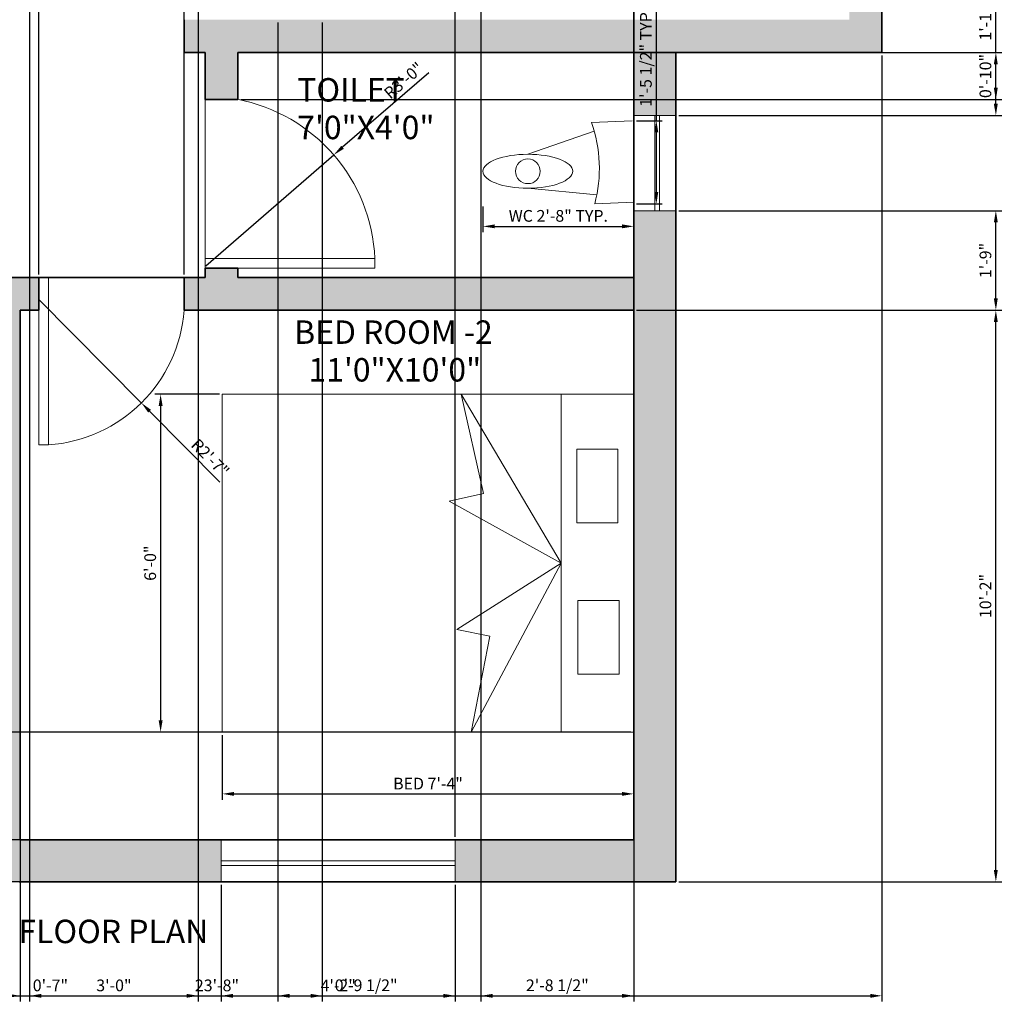
# Model space of a CAD drawing. Units: millimetres. Extents: x 2466 to 2817, y 2000 to 2512.
# Tile 2 of 4: x 2607 to 2817, y 2000 to 2210. Entities that reach past the tile are written whole.
import ezdxf

# ---------------------------------------------------------------- set-up
doc = ezdxf.new("R2010")
doc.units = ezdxf.units.MM
for name, color, linetype, lineweight in [('A-ANNO-DIMS', 2, 'Continuous', 13), ('A-ANNO-TEXT', 7, 'Continuous', 18), ('A-AREA-IDEN', 7, 'Continuous', 18), ('A-DOOR', 3, 'Continuous', 18), ('A-FLOR-FIXT', 9, 'Continuous', 18), ('A-FURN', 8, 'Continuous', 18), ('A-GLAZ', 5, 'Continuous', 18), ('A-WALL', 7, 'Continuous', 35), ('A-WALL-PATT', 8, 'Continuous', 13)]:
    doc.layers.add(name, color=color, linetype=linetype, lineweight=lineweight)
doc.styles.get("Standard").update_dxf_attribs({"font": 'arial.ttf'})
doc.dimstyles.new('ISO-25', dxfattribs={"dimtxt": 2.5, "dimasz": 2.5, "dimexe": 1.25, "dimexo": 0.625, "dimtad": 1, "dimdec": 0, "dimlunit": 3, "dimtxsty": 'Standard', "dimcen": 2.5, "dimadec": 0, "dimazin": 0, "dimtfac": 1, "dimtdec": 0, "dimtmove": 0, "dimatfit": 3, "dimfxl": 1, "dimarcsym": 0})

# ---------------------------------------------------------------- blocks, each defined once
blk = doc.blocks.new('MODERN BED')
at = {"color": 0}
for p, q in [((-79.02, 96.24), (0, 96.24)), ((-79.02, 0), (-79.02, 96.24)), ((0, 96.24), (0, 0)), ((0, 79.26), (-79.02, 79.26)), ((-39.51, 79.26), (-79.02, 55.87)), ((-53.99, 53.1), (-39.51, 79.26)), ((-39.51, 79.26), (0, 58.21)), ((-23.98, 54.83), (-39.51, 79.26)), ((-22.46, 62.6), (-23.98, 54.83)), ((0, 58.21), (-22.46, 62.6)), ((-79.02, 55.87), (-55.81, 61.13)), ((-55.81, 61.13), (-53.99, 53.1)), ((0, 0), (-79.02, 0))]:
    blk.add_line(p, q, dxfattribs=at)
for points in [[(-66.19, 92.55), (-48.93, 92.55), (-48.93, 82.91), (-66.19, 82.91)], [(-30.8, 92.85), (-13.54, 92.85), (-13.54, 83.2), (-30.8, 83.2)], [(-30.8, 92.85), (-13.54, 92.85), (-13.54, 83.2), (-30.8, 83.2)]]:
    blk.add_lwpolyline(points, close=True, dxfattribs=at)
blk = doc.blocks.new('*D10')
at = {"layer": 'A-ANNO-DIMS', "color": 0, "lineweight": -2, "transparency": 16777216}
for p, q in [((2746.56, 2482.15), (2467.98, 2482.15)), ((2469.23, 2479.65), (2469.23, 2028.65)), ((2746.56, 2026.15), (2467.98, 2026.15))]:
    blk.add_line(p, q, dxfattribs=at)
at = {"layer": 'A-ANNO-DIMS', "color": 0, "transparency": 16777216}
for points in [[(2468.82, 2479.65), (2469.65, 2479.65), (2469.23, 2482.15)], [(2468.82, 2028.65), (2469.65, 2028.65), (2469.23, 2026.15)]]:
    blk.add_solid(points, dxfattribs=at)
at = {"layer": 'Defpoints', "color": 0, "transparency": 16777216}
for p in [(2747.19, 2482.15), (2469.23, 2026.15), (2747.19, 2026.15)]:
    blk.add_point(p, dxfattribs=at)
at = {"layer": 'A-ANNO-DIMS', "color": 0, "transparency": 16777216, "insert": (2467.33, 2254.15), "char_height": 2.5, "attachment_point": 5, "rotation": 90}
blk.add_mtext("38'", dxfattribs=at)
blk = doc.blocks.new('WC-PLAN')
for p, q in [((23.15, 17.36), (31.83, 17.72)), ((23.74, 15.5), (9.57, 10.55)), ((24.29, 1.87), (9.58, 3.3)), ((32.19, 0.34), (23.86, 0))]:
    blk.add_line(p, q)
blk.add_circle((9.58, 6.93), 2.64)
blk.add_arc((-4.38, 7.53), 29.23, 345.0736, 19.6488)
blk.add_ellipse((9.58, 6.93), major_axis=(9.58, 0.01), ratio=0.378572)
blk = doc.blocks.new('WIN-BATH')
for p, q in [((4.5, 20.33), (4.5, 0)), ((5.5, 20.33), (5.5, 0))]:
    blk.add_line(p, q)
blk.add_lwpolyline([(9, 20.33), (0, 20.33), (0, 0), (9, 0)], close=True)
blk = doc.blocks.new('*D20')
at = {"layer": 'A-ANNO-DIMS', "color": 0, "lineweight": -2, "transparency": 16777216}
for p, q in [((2706, 2170.25), (2706, 2164.79)), ((2738.19, 2170.25), (2738.19, 2164.79)), ((2708.5, 2166.04), (2735.69, 2166.04))]:
    blk.add_line(p, q, dxfattribs=at)
at = {"layer": 'A-ANNO-DIMS', "color": 0, "transparency": 16777216}
for points in [[(2708.5, 2166.46), (2708.5, 2165.63), (2706, 2166.04)], [(2735.69, 2166.46), (2735.69, 2165.63), (2738.19, 2166.04)]]:
    blk.add_solid(points, dxfattribs=at)
at = {"layer": 'Defpoints', "color": 0, "transparency": 16777216}
for p in [(2706, 2170.87), (2738.19, 2170.87), (2738.19, 2166.04)]:
    blk.add_point(p, dxfattribs=at)
at = {"layer": 'A-ANNO-DIMS', "color": 0, "transparency": 16777216, "insert": (2722.09, 2167.96), "char_height": 2.5, "attachment_point": 5}
blk.add_mtext('WC 2\'-8" TYP.', dxfattribs=at)
blk = doc.blocks.new('*D21')
at = {"layer": 'A-ANNO-DIMS', "color": 0, "lineweight": -2, "transparency": 16777216}
for p, q in [((2743.02, 2188.59), (2743.02, 2213.17)), ((2738.81, 2188.59), (2744.27, 2188.59)), ((2743.02, 2173.37), (2743.02, 2186.09)), ((2738.81, 2170.87), (2744.27, 2170.87))]:
    blk.add_line(p, q, dxfattribs=at)
at = {"layer": 'A-ANNO-DIMS', "color": 0, "transparency": 16777216}
for points in [[(2742.6, 2186.09), (2743.43, 2186.09), (2743.02, 2188.59)], [(2742.6, 2173.37), (2743.43, 2173.37), (2743.02, 2170.87)]]:
    blk.add_solid(points, dxfattribs=at)
at = {"layer": 'Defpoints', "color": 0, "transparency": 16777216}
for p in [(2738.19, 2188.59), (2743.02, 2188.59), (2738.19, 2170.87)]:
    blk.add_point(p, dxfattribs=at)
at = {"layer": 'A-ANNO-DIMS', "color": 0, "transparency": 16777216, "insert": (2741.1, 2202.13), "char_height": 2.5, "attachment_point": 5, "rotation": 90}
blk.add_mtext('1\'-5 1/2" TYP.', dxfattribs=at)
blk = doc.blocks.new('*D22')
at = {"layer": 'A-ANNO-DIMS', "color": 0, "lineweight": -2, "transparency": 16777216}
for p, q in [((2650.34, 2057.48), (2650.34, 2043.67)), ((2738.19, 2057.48), (2738.19, 2043.67)), ((2652.84, 2044.92), (2735.69, 2044.92))]:
    blk.add_line(p, q, dxfattribs=at)
at = {"layer": 'A-ANNO-DIMS', "color": 0, "transparency": 16777216}
for points in [[(2652.84, 2045.34), (2652.84, 2044.51), (2650.34, 2044.92)], [(2735.69, 2045.34), (2735.69, 2044.51), (2738.19, 2044.92)]]:
    blk.add_solid(points, dxfattribs=at)
at = {"layer": 'Defpoints', "color": 0, "transparency": 16777216}
for p in [(2650.34, 2058.1), (2738.19, 2058.1), (2738.19, 2044.92)]:
    blk.add_point(p, dxfattribs=at)
at = {"layer": 'A-ANNO-DIMS', "color": 0, "transparency": 16777216, "insert": (2694.26, 2046.8), "char_height": 2.5, "attachment_point": 5}
blk.add_mtext('BED 7\'-4"', dxfattribs=at)
blk = doc.blocks.new('*D23')
at = {"layer": 'A-ANNO-DIMS', "color": 0, "lineweight": -2, "transparency": 16777216}
for p, q in [((2649.72, 2130.23), (2635.91, 2130.23)), ((2637.16, 2127.73), (2637.16, 2060.6)), ((2649.72, 2058.1), (2635.91, 2058.1))]:
    blk.add_line(p, q, dxfattribs=at)
at = {"layer": 'A-ANNO-DIMS', "color": 0, "transparency": 16777216}
for points in [[(2636.75, 2127.73), (2637.58, 2127.73), (2637.16, 2130.23)], [(2636.75, 2060.6), (2637.58, 2060.6), (2637.16, 2058.1)]]:
    blk.add_solid(points, dxfattribs=at)
at = {"layer": 'Defpoints', "color": 0, "transparency": 16777216}
for p in [(2650.34, 2130.23), (2637.16, 2058.1), (2650.34, 2058.1)]:
    blk.add_point(p, dxfattribs=at)
at = {"layer": 'A-ANNO-DIMS', "color": 0, "transparency": 16777216, "insert": (2635.26, 2094.16), "char_height": 2.5, "attachment_point": 5, "rotation": 90}
blk.add_mtext('6\'-0"', dxfattribs=at)
blk = doc.blocks.new('*D26')
at = {"layer": 'A-ANNO-DIMS', "color": 0, "lineweight": -2, "transparency": 16777216}
for p, q in [((2791.19, 2202.52), (2791.19, 2000.58)), ((2507.19, 2047.52), (2507.19, 2000.58)), ((2509.69, 2001.83), (2788.69, 2001.83))]:
    blk.add_line(p, q, dxfattribs=at)
at = {"layer": 'A-ANNO-DIMS', "color": 0, "transparency": 16777216}
for points in [[(2509.69, 2002.24), (2509.69, 2001.41), (2507.19, 2001.83)], [(2788.69, 2002.24), (2788.69, 2001.41), (2791.19, 2001.83)]]:
    blk.add_solid(points, dxfattribs=at)
at = {"layer": 'Defpoints', "color": 0, "transparency": 16777216}
for p in [(2791.19, 2203.15), (2507.19, 2048.15), (2791.19, 2001.83)]:
    blk.add_point(p, dxfattribs=at)
at = {"layer": 'A-ANNO-DIMS', "color": 0, "transparency": 16777216, "insert": (2649.19, 2003.73), "char_height": 2.5, "attachment_point": 5}
blk.add_mtext('23\'-8"', dxfattribs=at)
blk = doc.blocks.new('*D42')
at = {"layer": 'A-ANNO-DIMS', "color": 0, "lineweight": -2, "transparency": 16777216}
for p, q in [((2650.11, 2025.52), (2650.11, 2000.58)), ((2700.05, 2025.52), (2700.05, 2000.58)), ((2652.61, 2001.83), (2697.55, 2001.83))]:
    blk.add_line(p, q, dxfattribs=at)
at = {"layer": 'A-ANNO-DIMS', "color": 0, "transparency": 16777216}
for points in [[(2652.61, 2002.24), (2652.61, 2001.41), (2650.11, 2001.83)], [(2697.55, 2002.24), (2697.55, 2001.41), (2700.05, 2001.83)]]:
    blk.add_solid(points, dxfattribs=at)
at = {"layer": 'Defpoints', "color": 0, "transparency": 16777216}
for p in [(2650.11, 2026.15), (2700.05, 2026.15), (2700.05, 2001.83)]:
    blk.add_point(p, dxfattribs=at)
at = {"layer": 'A-ANNO-DIMS', "color": 0, "transparency": 16777216, "insert": (2675.08, 2003.71), "char_height": 2.5, "attachment_point": 5}
blk.add_mtext('4\'-2"', dxfattribs=at)
blk = doc.blocks.new('*D43')
at = {"layer": 'A-ANNO-DIMS', "color": 0, "lineweight": -2, "transparency": 16777216}
for p, q in [((2700.05, 2035.77), (2700.05, 2507.72)), ((2702.55, 2506.47), (2735.69, 2506.47)), ((2738.19, 2035.77), (2738.19, 2507.72))]:
    blk.add_line(p, q, dxfattribs=at)
at = {"layer": 'A-ANNO-DIMS', "color": 0, "transparency": 16777216}
for points in [[(2702.55, 2506.88), (2702.55, 2506.05), (2700.05, 2506.47)], [(2735.69, 2506.88), (2735.69, 2506.05), (2738.19, 2506.47)]]:
    blk.add_solid(points, dxfattribs=at)
at = {"layer": 'Defpoints', "color": 0, "transparency": 16777216}
for p in [(2738.19, 2506.47), (2700.05, 2035.15), (2738.19, 2035.15)]:
    blk.add_point(p, dxfattribs=at)
at = {"layer": 'A-ANNO-DIMS', "color": 0, "transparency": 16777216, "insert": (2719.12, 2508.37), "char_height": 2.5, "attachment_point": 5}
blk.add_mtext('3\'-2"', dxfattribs=at)
blk = doc.blocks.new('*D50')
at = {"layer": 'A-ANNO-DIMS', "color": 0, "lineweight": -2, "transparency": 16777216}
for p, q in [((2609.19, 2348.52), (2609.19, 2000.58)), ((2645.19, 2348.52), (2645.19, 2000.58)), ((2611.69, 2001.83), (2642.69, 2001.83))]:
    blk.add_line(p, q, dxfattribs=at)
at = {"layer": 'A-ANNO-DIMS', "color": 0, "transparency": 16777216}
for points in [[(2611.69, 2002.24), (2611.69, 2001.41), (2609.19, 2001.83)], [(2642.69, 2002.24), (2642.69, 2001.41), (2645.19, 2001.83)]]:
    blk.add_solid(points, dxfattribs=at)
at = {"layer": 'Defpoints', "color": 0, "transparency": 16777216}
for p in [(2609.19, 2349.15), (2645.19, 2349.15), (2645.19, 2001.83)]:
    blk.add_point(p, dxfattribs=at)
at = {"layer": 'A-ANNO-DIMS', "color": 0, "transparency": 16777216, "insert": (2627.19, 2003.73), "char_height": 2.5, "attachment_point": 5}
blk.add_mtext('3\'-0"', dxfattribs=at)
blk = doc.blocks.new('*D53')
at = {"layer": 'A-ANNO-DIMS', "color": 0, "lineweight": -2, "transparency": 16777216}
for p, q in [((2596.19, 2155.77), (2596.19, 2507.72)), ((2598.69, 2506.47), (2608.69, 2506.47)), ((2611.19, 2155.77), (2611.19, 2507.72))]:
    blk.add_line(p, q, dxfattribs=at)
at = {"layer": 'A-ANNO-DIMS', "color": 0, "transparency": 16777216}
for points in [[(2598.69, 2506.88), (2598.69, 2506.05), (2596.19, 2506.47)], [(2608.69, 2506.88), (2608.69, 2506.05), (2611.19, 2506.47)]]:
    blk.add_solid(points, dxfattribs=at)
at = {"layer": 'Defpoints', "color": 0, "transparency": 16777216}
for p in [(2611.19, 2506.47), (2596.19, 2155.15), (2611.19, 2155.15)]:
    blk.add_point(p, dxfattribs=at)
at = {"layer": 'A-ANNO-DIMS', "color": 0, "transparency": 16777216, "insert": (2603.69, 2508.37), "char_height": 2.5, "attachment_point": 5}
blk.add_mtext('1\'-3"', dxfattribs=at)
blk = doc.blocks.new('*D54')
at = {"layer": 'A-ANNO-DIMS', "color": 0, "lineweight": -2, "transparency": 16777216}
for p, q in [((2611.19, 2155.77), (2611.19, 2507.72)), ((2613.69, 2506.47), (2639.69, 2506.47)), ((2642.19, 2155.77), (2642.19, 2507.72))]:
    blk.add_line(p, q, dxfattribs=at)
at = {"layer": 'A-ANNO-DIMS', "color": 0, "transparency": 16777216}
for points in [[(2613.69, 2506.88), (2613.69, 2506.05), (2611.19, 2506.47)], [(2639.69, 2506.88), (2639.69, 2506.05), (2642.19, 2506.47)]]:
    blk.add_solid(points, dxfattribs=at)
at = {"layer": 'Defpoints', "color": 0, "transparency": 16777216}
for p in [(2642.19, 2506.47), (2611.19, 2155.15), (2642.19, 2155.15)]:
    blk.add_point(p, dxfattribs=at)
at = {"layer": 'A-ANNO-DIMS', "color": 0, "transparency": 16777216, "insert": (2626.69, 2508.35), "char_height": 2.5, "attachment_point": 5}
blk.add_mtext('2\'-7"', dxfattribs=at)
blk = doc.blocks.new('*D55')
at = {"layer": 'A-ANNO-DIMS', "color": 0, "lineweight": -2, "transparency": 16777216}
for p, q in [((2738.81, 2148.15), (2816.76, 2148.15)), ((2815.51, 2028.65), (2815.51, 2145.65)), ((2747.81, 2026.15), (2816.76, 2026.15))]:
    blk.add_line(p, q, dxfattribs=at)
at = {"layer": 'A-ANNO-DIMS', "color": 0, "transparency": 16777216}
for points in [[(2815.09, 2145.65), (2815.92, 2145.65), (2815.51, 2148.15)], [(2815.09, 2028.65), (2815.92, 2028.65), (2815.51, 2026.15)]]:
    blk.add_solid(points, dxfattribs=at)
at = {"layer": 'Defpoints', "color": 0, "transparency": 16777216}
for p in [(2738.19, 2148.15), (2815.51, 2148.15), (2747.19, 2026.15)]:
    blk.add_point(p, dxfattribs=at)
at = {"layer": 'A-ANNO-DIMS', "color": 0, "transparency": 16777216, "insert": (2813.61, 2087.15), "char_height": 2.5, "attachment_point": 5, "rotation": 90}
blk.add_mtext('10\'-2"', dxfattribs=at)
blk = doc.blocks.new('*D56')
at = {"layer": 'A-ANNO-DIMS', "color": 0, "lineweight": -2, "transparency": 16777216}
for p, q in [((2747.81, 2169.38), (2816.76, 2169.38)), ((2815.51, 2150.65), (2815.51, 2166.88)), ((2738.81, 2148.15), (2816.76, 2148.15))]:
    blk.add_line(p, q, dxfattribs=at)
at = {"layer": 'A-ANNO-DIMS', "color": 0, "transparency": 16777216}
for points in [[(2815.09, 2166.88), (2815.92, 2166.88), (2815.51, 2169.38)], [(2815.09, 2150.65), (2815.92, 2150.65), (2815.51, 2148.15)]]:
    blk.add_solid(points, dxfattribs=at)
at = {"layer": 'Defpoints', "color": 0, "transparency": 16777216}
for p in [(2747.19, 2169.38), (2815.51, 2169.38), (2738.19, 2148.15)]:
    blk.add_point(p, dxfattribs=at)
at = {"layer": 'A-ANNO-DIMS', "color": 0, "transparency": 16777216, "insert": (2813.61, 2158.76), "char_height": 2.5, "attachment_point": 5, "rotation": 90}
blk.add_mtext('1\'-9"', dxfattribs=at)
blk = doc.blocks.new('*D57')
at = {"layer": 'A-ANNO-DIMS', "color": 0, "lineweight": -2, "transparency": 16777216}
for p, q in [((2815.51, 2203.15), (2815.51, 2219.13)), ((2747.81, 2203.15), (2816.76, 2203.15)), ((2815.51, 2192.2), (2815.51, 2200.65)), ((2747.81, 2189.7), (2816.76, 2189.7))]:
    blk.add_line(p, q, dxfattribs=at)
at = {"layer": 'A-ANNO-DIMS', "color": 0, "transparency": 16777216}
for points in [[(2815.09, 2200.65), (2815.92, 2200.65), (2815.51, 2203.15)], [(2815.09, 2192.2), (2815.92, 2192.2), (2815.51, 2189.7)]]:
    blk.add_solid(points, dxfattribs=at)
at = {"layer": 'Defpoints', "color": 0, "transparency": 16777216}
for p in [(2747.19, 2203.15), (2815.51, 2203.15), (2747.19, 2189.7)]:
    blk.add_point(p, dxfattribs=at)
at = {"layer": 'A-ANNO-DIMS', "color": 0, "transparency": 16777216, "insert": (2813.59, 2212.39), "char_height": 2.5, "attachment_point": 5, "rotation": 90}
blk.add_mtext('1\'-1 1/2"', dxfattribs=at)
blk = doc.blocks.new('*D59')
at = {"layer": 'A-ANNO-DIMS', "color": 0, "lineweight": -2, "transparency": 16777216}
for p, q in [((2600.19, 2147.52), (2600.19, 2000.58)), ((2607.19, 2147.52), (2607.19, 2000.58)), ((2602.69, 2001.83), (2604.69, 2001.83)), ((2607.19, 2001.83), (2617.58, 2001.83))]:
    blk.add_line(p, q, dxfattribs=at)
at = {"layer": 'A-ANNO-DIMS', "color": 0, "transparency": 16777216}
for points in [[(2602.69, 2002.24), (2602.69, 2001.41), (2600.19, 2001.83)], [(2604.69, 2002.24), (2604.69, 2001.41), (2607.19, 2001.83)]]:
    blk.add_solid(points, dxfattribs=at)
at = {"layer": 'Defpoints', "color": 0, "transparency": 16777216}
for p in [(2600.19, 2148.15), (2607.19, 2148.15), (2607.19, 2001.83)]:
    blk.add_point(p, dxfattribs=at)
at = {"layer": 'A-ANNO-DIMS', "color": 0, "transparency": 16777216, "insert": (2613.63, 2003.73), "char_height": 2.5, "attachment_point": 5}
blk.add_mtext('0\'-7"', dxfattribs=at)
blk = doc.blocks.new('*D62')
at = {"layer": 'A-ANNO-DIMS', "color": 0, "lineweight": -2, "transparency": 16777216}
for p, q in [((2654.3, 2203.15), (2816.76, 2203.15)), ((2815.51, 2195.61), (2815.51, 2200.65)), ((2654.3, 2193.11), (2816.76, 2193.11))]:
    blk.add_line(p, q, dxfattribs=at)
at = {"layer": 'A-ANNO-DIMS', "color": 0, "transparency": 16777216}
for points in [[(2815.09, 2200.65), (2815.92, 2200.65), (2815.51, 2203.15)], [(2815.09, 2195.61), (2815.92, 2195.61), (2815.51, 2193.11)]]:
    blk.add_solid(points, dxfattribs=at)
at = {"layer": 'Defpoints', "color": 0, "transparency": 16777216}
for p in [(2653.68, 2203.15), (2815.51, 2203.15), (2653.68, 2193.11)]:
    blk.add_point(p, dxfattribs=at)
at = {"layer": 'A-ANNO-DIMS', "color": 0, "transparency": 16777216, "insert": (2813.61, 2198.13), "char_height": 2.5, "attachment_point": 5, "rotation": 90}
blk.add_mtext('0\'-10"', dxfattribs=at)
blk = doc.blocks.new('*D63')
at = {"layer": 'A-ANNO-DIMS', "color": 0, "lineweight": -2, "transparency": 16777216}
for p, q in [((2662.19, 2209.52), (2662.19, 2000.58)), ((2671.69, 2209.52), (2671.69, 2000.58)), ((2664.69, 2001.83), (2669.19, 2001.83)), ((2671.69, 2001.83), (2687.91, 2001.83))]:
    blk.add_line(p, q, dxfattribs=at)
at = {"layer": 'A-ANNO-DIMS', "color": 0, "transparency": 16777216}
for points in [[(2664.69, 2002.24), (2664.69, 2001.41), (2662.19, 2001.83)], [(2669.19, 2002.24), (2669.19, 2001.41), (2671.69, 2001.83)]]:
    blk.add_solid(points, dxfattribs=at)
at = {"layer": 'Defpoints', "color": 0, "transparency": 16777216}
for p in [(2662.19, 2210.15), (2671.69, 2210.15), (2671.69, 2001.83)]:
    blk.add_point(p, dxfattribs=at)
at = {"layer": 'A-ANNO-DIMS', "color": 0, "transparency": 16777216, "insert": (2681.05, 2003.75), "char_height": 2.5, "attachment_point": 5}
blk.add_mtext('0\'-9 1/2"', dxfattribs=at)
blk = doc.blocks.new('*D67')
at = {"layer": 'A-ANNO-DIMS', "color": 0, "lineweight": -2, "transparency": 16777216}
for p, q in [((2705.56, 2472.66), (2705.56, 2000.58)), ((2738.19, 2472.52), (2738.19, 2000.58)), ((2708.06, 2001.83), (2735.69, 2001.83))]:
    blk.add_line(p, q, dxfattribs=at)
at = {"layer": 'A-ANNO-DIMS', "color": 0, "transparency": 16777216}
for points in [[(2708.06, 2002.24), (2708.06, 2001.41), (2705.56, 2001.83)], [(2735.69, 2002.24), (2735.69, 2001.41), (2738.19, 2001.83)]]:
    blk.add_solid(points, dxfattribs=at)
at = {"layer": 'Defpoints', "color": 0, "transparency": 16777216}
for p in [(2705.56, 2473.28), (2738.19, 2473.15), (2738.19, 2001.83)]:
    blk.add_point(p, dxfattribs=at)
at = {"layer": 'A-ANNO-DIMS', "color": 0, "transparency": 16777216, "insert": (2721.87, 2003.75), "char_height": 2.5, "attachment_point": 5}
blk.add_mtext('2\'-8 1/2"', dxfattribs=at)
blk = doc.blocks.new('*D68')
at = {"layer": 'A-ANNO-DIMS', "color": 0, "lineweight": -2, "transparency": 16777216}
for p, q in [((2737.56, 2058.1), (2481.62, 2058.1)), ((2482.87, 2037.65), (2482.87, 2055.6)), ((2737.56, 2035.15), (2481.62, 2035.15))]:
    blk.add_line(p, q, dxfattribs=at)
at = {"layer": 'A-ANNO-DIMS', "color": 0, "transparency": 16777216}
for points in [[(2482.45, 2055.6), (2483.28, 2055.6), (2482.87, 2058.1)], [(2482.45, 2037.65), (2483.28, 2037.65), (2482.87, 2035.15)]]:
    blk.add_solid(points, dxfattribs=at)
at = {"layer": 'Defpoints', "color": 0, "transparency": 16777216}
for p in [(2482.87, 2058.1), (2738.19, 2058.1), (2738.19, 2035.15)]:
    blk.add_point(p, dxfattribs=at)
at = {"layer": 'A-ANNO-DIMS', "color": 0, "transparency": 16777216, "insert": (2480.99, 2046.62), "char_height": 2.5, "attachment_point": 5, "rotation": 90}
blk.add_mtext('1\'-11"', dxfattribs=at)
blk = doc.blocks.new('*D75')
at = {"layer": 'A-ANNO-DIMS', "color": 0, "lineweight": -2, "transparency": 16777216}
for p, q in [((2694.41, 2198.84), (2676.01, 2182.92)), ((2646.79, 2157.63), (2674.12, 2181.28))]:
    blk.add_line(p, q, dxfattribs=at)
at = {"layer": 'A-ANNO-DIMS', "color": 0, "transparency": 16777216}
blk.add_solid([(2675.74, 2183.23), (2676.28, 2182.6), (2674.12, 2181.28)], dxfattribs=at)
at = {"layer": 'Defpoints', "color": 0, "transparency": 16777216}
for p in [(2674.12, 2181.28), (2646.79, 2157.63)]:
    blk.add_point(p, dxfattribs=at)
at = {"layer": 'A-ANNO-DIMS', "color": 0, "transparency": 16777216, "insert": (2689.28, 2196.91), "char_height": 2.5, "attachment_point": 5, "rotation": 40.8737}
blk.add_mtext('R3\'-0"', dxfattribs=at)
blk = doc.blocks.new('*D79')
at = {"layer": 'A-ANNO-DIMS', "color": 0, "lineweight": -2, "transparency": 16777216}
for p, q in [((2611.1, 2150.52), (2633.04, 2128.38)), ((2649.83, 2111.43), (2634.8, 2126.6))]:
    blk.add_line(p, q, dxfattribs=at)
at = {"layer": 'A-ANNO-DIMS', "color": 0, "transparency": 16777216}
blk.add_solid([(2635.1, 2126.89), (2634.51, 2126.31), (2633.04, 2128.38)], dxfattribs=at)
at = {"layer": 'Defpoints', "color": 0, "transparency": 16777216}
for p in [(2611.1, 2150.52), (2633.04, 2128.38)]:
    blk.add_point(p, dxfattribs=at)
at = {"layer": 'A-ANNO-DIMS', "color": 0, "transparency": 16777216, "insert": (2647.54, 2116.41), "char_height": 2.5, "attachment_point": 5, "rotation": 314.7339}
blk.add_mtext('R2\'-7"', dxfattribs=at)

msp = doc.modelspace()

# ---------------------------------------------------------------- hatches: boundary and pattern name
at = {"layer": 'A-WALL-PATT'}
h = msp.add_hatch(color=256, dxfattribs=at)
h.dxf.hatch_style = 1
h.paths.add_polyline_path([(2791.19, 2301.15), (2747.19, 2301.15), (2747.19, 2294.15), (2784.19, 2294.15), (2784.19, 2279.03), (2791.19, 2279.03)])
h.paths.add_polyline_path([(2791.19, 2216.9), (2784.19, 2216.9), (2784.19, 2210.15), (2662.19, 2210.15), (2647.19, 2210.15), (2645.19, 2210.15), (2642.19, 2210.15), (2642.19, 2203.15), (2646.68, 2203.15), (2646.68, 2193.15), (2653.68, 2193.15), (2653.68, 2203.15), (2654.69, 2203.15), (2662.19, 2203.15), (2791.19, 2203.15)])
h = msp.add_hatch(color=256, dxfattribs=at)
h.dxf.hatch_style = 1
h.paths.add_polyline_path([(2747.19, 2203.15), (2738.19, 2203.15), (2738.19, 2189.7), (2747.19, 2189.7)])
h = msp.add_hatch(color=256, dxfattribs=at)
h.dxf.hatch_style = 1
h.paths.add_polyline_path([(2747.19, 2169.38), (2738.19, 2169.38), (2738.19, 2035.15), (2700.05, 2035.15), (2700.05, 2026.15), (2747.19, 2026.15)])
h = msp.add_hatch(color=256, dxfattribs=at)
h.dxf.hatch_style = 1
h.paths.add_polyline_path([(2516.19, 2159.02), (2507.19, 2159.02), (2507.19, 2119.17), (2516.19, 2119.17)])
h.paths.add_polyline_path([(2516.19, 2068.93), (2507.19, 2068.93), (2507.19, 2048.15), (2516.19, 2048.15), (2562.24, 2048.15), (2562.24, 2055.15), (2551.24, 2055.15), (2516.19, 2055.15)])
h.paths.add_polyline_path([(2607.19, 2148.15), (2611.19, 2148.15), (2611.19, 2155.15), (2596.19, 2155.15), (2596.19, 2148.15), (2600.19, 2148.15), (2600.19, 2055.15), (2598.12, 2055.15), (2598.12, 2048.15), (2600.19, 2048.15), (2600.19, 2035.15), (2600.19, 2026.15), (2606.96, 2026.15), (2650.11, 2026.15), (2650.11, 2035.15), (2607.19, 2035.15)])
h = msp.add_hatch(color=256, dxfattribs=at)
h.dxf.hatch_style = 1
h.paths.add_polyline_path([(2738.19, 2155.15), (2653.68, 2155.15), (2653.68, 2157.15), (2646.68, 2157.15), (2646.68, 2155.15), (2642.19, 2155.15), (2642.19, 2148.15), (2738.19, 2148.15)])

# ---------------------------------------------------------------- linework, layer by layer
at = {"layer": 'A-DOOR'}
for p, q in [((2646.7, 2157.15), (2646.68, 2193.15)), ((2682.9, 2159.15), (2646.7, 2159.15)), ((2646.7, 2159.15), (2646.7, 2157.15)), ((2653.68, 2157.15), (2682.9, 2157.15)), ((2682.9, 2157.15), (2682.9, 2159.15)), ((2613.19, 2119.42), (2613.19, 2155.15)), ((2611.19, 2148.15), (2611.19, 2119.42)), ((2611.19, 2119.42), (2613.19, 2119.42))]:
    msp.add_line(p, q, dxfattribs=at)
for centre, radius, start, end in [((2646.79, 2157.63), 36.15, 2.4119, 79.3368), ((2611.1, 2150.52), 31.18, 273.8392, 355.6301)]:
    msp.add_arc(centre, radius, start, end, dxfattribs=at)
at = {"layer": 'A-GLAZ'}
for p, q in [((2650.11, 2035.15), (2650.11, 2026.15)), ((2700.05, 2035.15), (2650.11, 2035.15)), ((2700.05, 2026.15), (2700.05, 2035.15)), ((2700.05, 2030.65), (2650.11, 2030.65)), ((2700.05, 2029.65), (2650.11, 2029.65)), ((2650.11, 2026.15), (2700.05, 2026.15))]:
    msp.add_line(p, q, dxfattribs=at)
at = {"layer": 'A-WALL'}
for p, q in [((2791.19, 2301.15), (2791.19, 2203.15)), ((2642.19, 2210.15), (2642.19, 2203.15)), ((2642.19, 2203.15), (2646.68, 2203.15)), ((2646.68, 2203.15), (2646.68, 2193.11)), ((2653.68, 2203.15), (2653.68, 2193.11)), ((2654.69, 2203.15), (2653.68, 2203.15)), ((2662.19, 2203.15), (2654.69, 2203.15)), ((2791.19, 2203.15), (2662.19, 2203.15)), ((2738.19, 2203.15), (2738.19, 2035.15)), ((2747.19, 2203.15), (2747.19, 2026.15)), ((2646.68, 2193.15), (2653.68, 2193.15)), ((2646.68, 2155.15), (2646.68, 2157.15)), ((2646.68, 2157.15), (2653.68, 2157.15)), ((2653.68, 2157.15), (2653.68, 2155.15)), ((2642.19, 2155.15), (2516.19, 2155.15)), ((2611.19, 2148.15), (2611.19, 2155.15)), ((2642.19, 2155.15), (2646.68, 2155.15)), ((2642.19, 2155.15), (2642.19, 2148.15)), ((2653.68, 2155.15), (2738.19, 2155.15)), ((2611.19, 2148.15), (2607.19, 2148.15)), ((2607.19, 2035.15), (2607.19, 2148.15)), ((2642.19, 2148.15), (2738.19, 2148.15)), ((2738.19, 2035.15), (2607.19, 2035.15)), ((2747.19, 2026.15), (2606.96, 2026.15))]:
    msp.add_line(p, q, dxfattribs=at)

# ---------------------------------------------------------------- block references
at = {"layer": 'A-FLOR-FIXT'}
msp.add_blockref('WC-PLAN', (2706, 2170.87), dxfattribs=at)
at = {"layer": 'A-FURN', "xscale": 0.9127362200850963, "yscale": 0.9127362200850963, "zscale": 0.9127362200850963, "rotation": 270}
msp.add_blockref('MODERN BED', (2650.34, 2058.1), dxfattribs=at)
at = {"layer": 'A-GLAZ'}
msp.add_blockref('WIN-BATH', (2738.19, 2169.38), dxfattribs=at)

# ---------------------------------------------------------------- texts
at = {"layer": 'A-ANNO-TEXT'}
msp.add_text('GROUND FLOOR PLAN', height=5, dxfattribs=at).set_placement((2576.64, 2013.07))
at = {"layer": 'A-AREA-IDEN'}
for s, p in [('TOILET', (2666.34, 2192.68)), ('7\'0"X4\'0"', (2666.34, 2184.65)), ('BED ROOM -2', (2665.68, 2140.97)), ('  11\'0"X10\'0"', (2665.68, 2132.93))]:
    msp.add_text(s, height=5, dxfattribs=at).set_placement(p)

# ---------------------------------------------------------------- dimensions: what is measured, and where the dimension line sits
at = {"layer": 'A-ANNO-DIMS'}
for base, p1, p2, picture, middle in [((2611.19, 2506.47), (2596.19, 2155.15), (2611.19, 2155.15), '*D53', (2603.69, 2508.37)), ((2642.19, 2506.47), (2611.19, 2155.15), (2642.19, 2155.15), '*D54', (2626.69, 2508.35)), ((2738.19, 2506.47), (2700.05, 2035.15), (2738.19, 2035.15), '*D43', (2719.12, 2508.37)), ((2738.19, 2001.83), (2705.56, 2473.28), (2738.19, 2473.15), '*D67', (2721.87, 2003.75)), ((2645.19, 2001.83), (2609.19, 2349.15), (2645.19, 2349.15), '*D50', (2627.19, 2003.73)), ((2671.69, 2001.83), (2662.19, 2210.15), (2671.69, 2210.15), '*D63', (2681.05, 2003.75)), ((2791.19, 2001.83), (2507.19, 2048.15), (2791.19, 2203.15), '*D26', (2649.19, 2003.73)), ((2607.19, 2001.83), (2600.19, 2148.15), (2607.19, 2148.15), '*D59', (2613.63, 2003.73)), ((2700.05, 2001.83), (2650.11, 2026.15), (2700.05, 2026.15), '*D42', (2675.08, 2003.71))]:
    dim = msp.add_linear_dim(base=base, p1=p1, p2=p2, dimstyle='ISO-25', override={"dimdec": 1, "dimlfac": 1, "dimrnd": 0, "dimzin": 1, "dimdsep": 46, "dimlunit": 4, "dimfrac": 2}, dxfattribs=at)
    dim.commit()
    dim.dimension.update_dxf_attribs({"geometry": picture, "text_midpoint": middle})
for base, p1, p2, angle, override, picture, middle in [((2469.23, 2026.15), (2747.19, 2482.15), (2747.19, 2026.15), 90, {"dimclrd": 0, "dimclre": 0, "dimclrt": 0}, '*D10', (2467.33, 2254.15)), ((2815.5068, 2203.1479), (2747.1868, 2189.7042), (2747.1868, 2203.1479), 90, {"dimdec": 1, "dimlfac": 1, "dimrnd": 0, "dimzin": 1, "dimdsep": 46, "dimlunit": 4, "dimfrac": 2}, '*D57', (2813.5892, 2212.3908)), ((2815.51, 2203.15), (2653.68, 2193.11), (2653.68, 2203.15), 90, {"dimdec": 1, "dimlfac": 1, "dimrnd": 0, "dimzin": 1, "dimdsep": 46, "dimlunit": 4, "dimfrac": 2}, '*D62', (2813.61, 2198.13)), ((2815.51, 2169.38), (2738.19, 2148.15), (2747.19, 2169.38), 90, {"dimdec": 1, "dimlfac": 1, "dimrnd": 0, "dimzin": 1, "dimdsep": 46, "dimlunit": 4, "dimfrac": 2}, '*D56', (2813.61, 2158.76)), ((2815.51, 2148.15), (2747.19, 2026.15), (2738.19, 2148.15), 90, {"dimdec": 1, "dimlfac": 1, "dimrnd": 0, "dimzin": 1, "dimdsep": 46, "dimlunit": 4, "dimfrac": 2}, '*D55', (2813.61, 2087.15)), ((2637.16, 2058.1), (2650.34, 2130.23), (2650.34, 2058.1), 270, {"dimdec": 1, "dimlfac": 1, "dimrnd": 0, "dimzin": 1, "dimdsep": 46, "dimlunit": 4, "dimfrac": 2}, '*D23', (2635.26, 2094.16)), ((2482.8668, 2058.1003), (2738.1868, 2035.1479), (2738.1868, 2058.1003), 90, {"dimdec": 1, "dimlfac": 1, "dimrnd": 0, "dimzin": 1, "dimdsep": 46, "dimlunit": 4, "dimfrac": 2}, '*D68', (2480.9867, 2046.6241))]:
    dim = msp.add_linear_dim(base=base, p1=p1, p2=p2, angle=angle, dimstyle='ISO-25', override=override, dxfattribs=at)
    dim.commit()
    dim.dimension.update_dxf_attribs({"geometry": picture, "text_midpoint": middle})
dim = msp.add_linear_dim(base=(2743.02, 2188.59), p1=(2738.19, 2170.87), p2=(2738.19, 2188.59), angle=90, text='<> TYP.', dimstyle='ISO-25', override={"dimdec": 1, "dimlfac": 1, "dimrnd": 0, "dimzin": 1, "dimdsep": 46, "dimlunit": 4, "dimfrac": 2}, dxfattribs=at)
dim.commit()
dim.dimension.update_dxf_attribs({"geometry": '*D21', "text_midpoint": (2741.1, 2202.13)})
for center, mpoint, picture, middle in [((2646.79, 2157.63), (2674.12, 2181.28), '*D75', (2690.52, 2195.47)), ((2611.1, 2150.52), (2633.04, 2128.38), '*D79', (2646.21, 2115.09))]:
    dim = msp.add_radius_dim(center=center, mpoint=mpoint, dimstyle='ISO-25', override={"dimdec": 1, "dimlfac": 1, "dimrnd": 0, "dimzin": 1, "dimdsep": 46, "dimlunit": 4, "dimfrac": 2}, dxfattribs=at)
    dim.commit()
    dim.dimension.update_dxf_attribs({"geometry": picture, "text_midpoint": middle, "dimtype": 164})
for base, p1, p2, text, picture, middle in [((2738.19, 2166.04), (2706, 2170.87), (2738.19, 2170.87), 'WC <> TYP.', '*D20', (2722.09, 2167.96)), ((2738.1868, 2044.9235), (2650.3413, 2058.1003), (2738.1868, 2058.1003), 'BED <>', '*D22', (2694.264, 2046.7994))]:
    dim = msp.add_linear_dim(base=base, p1=p1, p2=p2, text=text, dimstyle='ISO-25', override={"dimdec": 1, "dimlfac": 1, "dimrnd": 0, "dimzin": 1, "dimdsep": 46, "dimlunit": 4, "dimfrac": 2}, dxfattribs=at)
    dim.commit()
    dim.dimension.update_dxf_attribs({"geometry": picture, "text_midpoint": middle})

doc.saveas('drawing.dxf')
